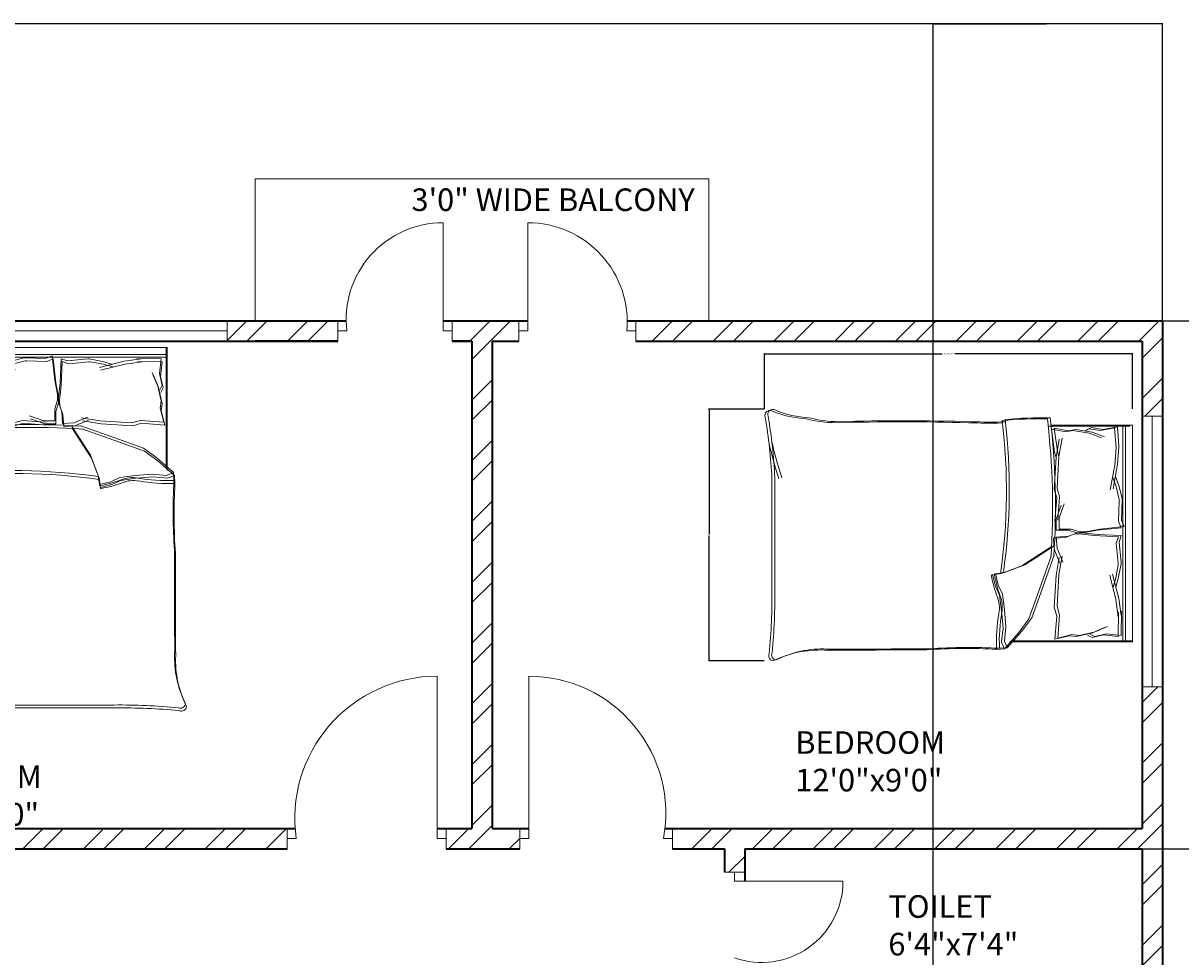
# Model space of a CAD drawing. Units: inches. Extents: x 2165 to 3042, y 1626 to 2968.
# Tile 9 of 11: x 2633 to 2889, y 2191 to 2398. Entities that reach past the tile are written whole.
import ezdxf

# ---------------------------------------------------------------- set-up
doc = ezdxf.new("R2010")
doc.units = ezdxf.units.IN
for name, color, linetype, lineweight in [('A-ANNO-DIMS', 2, 'Continuous', 18), ('A-AREA-IDEN', 7, 'Continuous', 18), ('A-DOOR', 3, 'Continuous', 18), ('A-FLOR-BALC', 7, 'Continuous', 18), ('A-FURN', 8, 'Continuous', 13), ('A-GLAZ', 4, 'Continuous', 18), ('A-WALL', 7, 'Continuous', 35), ('A-WALL-PATT', 252, 'Continuous', 13)]:
    doc.layers.add(name, color=color, linetype=linetype, lineweight=lineweight)
doc.styles.get("Standard").update_dxf_attribs({"font": 'arial.ttf'})
doc.dimstyles.get("Standard").update_dxf_attribs({"dimtxt": 0.18, "dimasz": 0.18, "dimexe": 0.18, "dimexo": 0.0625, "dimgap": 0.09, "dimtad": 0, "dimtih": 1, "dimtoh": 1, "dimdec": 4, "dimzin": 0, "dimdsep": 46, "dimtxsty": 'Standard', "dimcen": 0.09, "dimadec": 0, "dimazin": 0, "dimtfac": 1, "dimtdec": 4, "dimtofl": 0, "dimtmove": 0, "dimatfit": 3, "dimfxl": 1, "dimtolj": 1, "dimtzin": 0, "dimarcsym": 0})

# ---------------------------------------------------------------- blocks, each defined once
blk = doc.blocks.new('BED-DOUBLE')
for p, q in [((0, 51.27), (0, 51.49)), ((0, 51.49), (0.64, 51.49)), ((0.64, 51.49), (27.25, 51.49)), ((0.64, 51.49), (27.25, 51.49)), ((2.17, 3.7), (2.17, 51.49)), ((2.17, 3.7), (2.17, 51.49)), ((27.75, 52.87), (24.5, 49.16)), ((27.75, 52.87), (24.5, 49.16)), ((28.39, 53.1), (25.14, 49.39)), ((28.39, 53.1), (25.14, 49.39)), ((29.49, 52.95), (27.75, 52.87, 3.87)), ((29.49, 52.95), (27.75, 52.87, 3.87)), ((28.37, 51.33), (27.75, 52.87)), ((28.37, 51.33), (27.75, 52.87)), ((28.06, 48.23), (28.37, 51.33)), ((28.06, 48.23), (28.37, 51.33)), ((30.13, 53.18), (28.39, 53.1, 3.87)), ((30.13, 53.18), (28.39, 53.1, 3.87)), ((29, 51.56), (28.39, 53.1)), ((29, 51.56), (28.39, 53.1)), ((28.7, 48.46), (29, 51.56)), ((28.7, 48.46), (29, 51.56)), ((0, 51.27), (26.61, 51.27)), ((0, 51.27), (26.61, 51.27)), ((0, 51.27), (0, 3.48)), ((1.53, 3.48), (1.53, 51.27)), ((1.53, 3.47), (1.53, 51.27)), ((2.56, 50.11), (2.46, 44.71)), ((2.56, 50.11), (2.46, 44.71)), ((2.56, 50.11), (5.77, 49.73)), ((2.56, 50.11), (5.77, 49.73)), ((3.2, 50.34), (3.1, 44.94)), ((3.2, 50.34), (3.1, 44.94)), ((3.2, 50.34), (6.41, 49.96)), ((3.2, 50.34), (6.41, 49.96)), ((8.26, 49.31), (5.58, 48.13)), ((8.26, 49.31), (5.58, 48.13)), ((5.77, 49.73), (8.34, 50.33)), ((5.77, 49.73), (8.34, 50.33)), ((8.9, 49.54), (6.22, 48.36)), ((8.9, 49.54), (6.22, 48.36)), ((6.41, 49.96), (8.98, 50.56)), ((6.41, 49.96), (8.98, 50.56)), ((11.83, 50.11), (8.26, 49.31)), ((11.83, 50.11), (8.26, 49.31)), ((8.34, 50.33), (9.38, 49.81)), ((8.34, 50.33), (9.38, 49.81)), ((12.47, 50.34), (8.9, 49.54)), ((12.47, 50.34), (8.9, 49.54)), ((8.98, 50.56), (10.02, 50.04)), ((8.98, 50.56), (10.02, 50.04)), ((13.43, 49.92), (11.83, 50.11)), ((13.43, 49.92), (11.83, 50.11)), ((14.07, 50.15), (12.47, 50.34)), ((14.07, 50.15), (12.47, 50.34)), ((16.57, 50.7), (13.43, 49.92)), ((16.57, 50.7), (13.43, 49.92)), ((17.21, 50.93), (14.07, 50.15)), ((17.21, 50.93), (14.07, 50.15)), ((16.17, 45.57), (16.57, 50.7)), ((16.17, 45.57), (16.57, 50.7)), ((16.81, 45.79), (17.21, 50.93)), ((16.81, 45.79), (17.21, 50.93)), ((24.5, 49.16), (22.33, 46.22)), ((24.5, 49.16), (22.33, 46.22)), ((25.14, 49.39), (22.97, 46.45)), ((25.14, 49.39), (22.97, 46.45)), ((22.33, 46.22), (20.32, 40.64)), ((22.33, 46.22), (20.32, 40.64)), ((22.97, 46.45), (20.96, 40.87)), ((22.97, 46.45), (20.96, 40.87)), ((28.37, 44.36), (28.06, 48.23)), ((28.37, 44.36), (28.06, 48.23)), ((29, 44.59), (28.7, 48.46)), ((29, 44.59), (28.7, 48.46)), ((2.46, 44.71), (2.54, 45.71)), ((2.46, 44.71), (2.54, 45.71)), ((2.54, 45.71), (3.07, 41.91)), ((2.54, 45.71), (3.07, 41.91)), ((3.1, 44.94), (3.18, 45.94)), ((3.1, 44.94), (3.18, 45.94)), ((3.18, 45.94), (3.71, 42.14)), ((3.18, 45.94), (3.71, 42.14)), ((16.73, 43.61), (16.17, 45.57)), ((16.73, 43.61), (16.17, 45.57)), ((16.3, 36.6), (16.73, 43.61)), ((16.3, 36.6), (16.73, 43.61)), ((17.37, 43.83), (16.81, 45.79)), ((17.37, 43.83), (16.81, 45.79)), ((16.93, 36.82), (17.37, 43.83)), ((16.93, 36.82), (17.37, 43.83)), ((28.83, 40.95), (28.37, 44.36)), ((28.83, 40.95), (28.37, 44.36)), ((29.47, 41.18), (29, 44.59)), ((29.47, 41.18), (29, 44.59)), ((3.07, 41.91), (4.42, 36.5)), ((3.07, 41.91), (4.42, 36.49)), ((3.71, 42.14), (5.06, 36.72)), ((3.71, 42.14), (5.06, 36.72)), ((30.4, 39.17), (29.47, 41.18)), ((30.4, 39.17), (29.47, 41.18)), ((3.67, 39.2), (3.08, 37.14)), ((3.67, 39.2), (3.08, 37.13)), ((4.31, 39.43), (3.72, 37.36)), ((4.31, 39.43), (3.72, 37.36)), ((20.32, 40.64), (17.38, 32.31)), ((20.32, 40.64), (17.38, 32.31)), ((20.96, 40.87), (18.02, 32.53)), ((20.96, 40.87), (18.02, 32.53)), ((29.76, 38.94), (28.83, 40.95)), ((29.76, 38.94), (28.83, 40.95)), ((30.38, 36.46), (29.76, 38.94)), ((30.38, 36.46), (29.76, 38.94)), ((31.02, 36.69), (30.4, 39.17)), ((31.02, 36.69), (30.4, 39.17)), ((79.25, 15.06), (79.25, 39.68)), ((79.25, 15.06), (79.25, 39.68)), ((79.88, 15.29), (79.88, 39.91)), ((79.88, 15.29), (79.88, 39.91)), ((3.08, 37.14), (2.54, 34.2)), ((3.08, 37.13), (2.54, 34.2)), ((3.72, 37.36), (3.18, 34.43)), ((3.72, 37.36), (3.18, 34.43)), ((15.63, 32.56), (16.3, 36.6)), ((15.63, 32.56), (16.3, 36.6)), ((16.27, 32.79), (16.93, 36.82)), ((16.27, 32.79), (16.93, 36.82)), ((23.88, 34.45), (28.37, 36.15)), ((23.88, 34.45), (28.37, 36.15)), ((24.52, 34.68), (29, 36.38)), ((24.52, 34.68), (29, 36.38)), ((28.37, 36.15), (30.38, 36.46)), ((28.37, 36.15), (30.38, 36.46)), ((29, 36.38), (31.02, 36.69)), ((29, 36.38), (31.02, 36.69)), ((2.54, 34.2), (2.56, 33.88)), ((2.54, 34.2), (2.56, 33.88)), ((2.56, 33.88), (2.98, 29.46)), ((2.56, 33.88), (2.98, 29.46)), ((3.18, 34.43), (3.2, 34.11)), ((3.18, 34.43), (3.2, 34.11)), ((3.2, 34.11), (3.62, 29.68)), ((3.2, 34.11), (3.62, 29.68)), ((16.74, 30.75), (15.46, 33.82)), ((16.74, 30.75), (15.46, 33.82)), ((17.38, 30.98), (16.09, 34.05)), ((17.38, 30.98), (16.09, 34.05)), ((17.38, 30.26), (23.88, 34.45)), ((17.38, 30.26), (23.88, 34.45)), ((18.02, 30.49), (24.52, 34.68)), ((18.02, 30.49), (24.52, 34.68)), ((17.53, 28.53), (17.38, 30.98)), ((17.53, 28.53), (17.38, 30.98)), ((2.98, 29.46), (2.49, 27.98)), ((2.98, 29.46), (2.49, 27.98)), ((3.62, 29.68), (3.13, 28.21)), ((3.62, 29.68), (3.13, 28.21)), ((13.02, 27.66), (14.86, 28.36)), ((13.02, 27.66), (14.86, 28.36)), ((14.22, 28.13), (16.89, 28.3)), ((14.22, 28.13), (16.89, 28.3)), ((14.86, 28.36), (17.53, 28.53)), ((14.86, 28.36), (17.53, 28.53)), ((16.89, 28.3), (16.74, 30.75)), ((16.89, 28.3), (16.74, 30.75)), ((1.87, 25.98), (7.22, 26.56)), ((1.87, 25.98), (7.22, 26.56)), ((2.45, 24.54), (1.87, 25.98)), ((2.45, 24.54), (1.87, 25.98)), ((2.49, 27.98), (7.87, 27.73)), ((2.49, 27.98), (7.87, 27.73)), ((2.51, 26.21), (7.86, 26.79)), ((2.51, 26.21), (7.86, 26.79)), ((3.09, 24.77), (2.51, 26.21)), ((3.09, 24.77), (2.51, 26.21)), ((3.13, 28.21), (8.51, 27.96)), ((3.13, 28.21), (8.51, 27.96)), ((7.22, 26.56), (10.4, 27.14)), ((7.22, 26.56), (10.4, 27.14)), ((7.86, 26.79), (11.04, 27.37)), ((7.86, 26.79), (11.04, 27.37)), ((7.87, 27.73), (11.08, 27.35)), ((7.87, 27.73), (11.08, 27.35)), ((8.51, 27.96), (11.72, 27.58)), ((8.51, 27.96), (11.72, 27.58)), ((10.4, 27.14), (11.7, 27.14)), ((10.4, 27.14), (11.7, 27.14)), ((11.04, 27.37), (12.34, 27.37)), ((11.04, 27.37), (12.34, 27.37)), ((11.08, 27.35), (12.38, 27.44)), ((11.08, 27.35), (12.38, 27.44)), ((11.7, 27.14), (13.58, 26.56)), ((11.7, 27.14), (13.58, 26.56)), ((11.72, 27.58), (13.02, 27.66)), ((11.72, 27.58), (13.02, 27.66)), ((12.34, 27.37), (14.22, 26.79)), ((12.34, 27.37), (14.22, 26.79)), ((12.38, 27.44), (14.22, 28.13)), ((12.38, 27.44), (14.22, 28.13)), ((13.58, 26.56), (16.26, 26.56)), ((13.58, 26.56), (16.26, 26.56)), ((14.22, 26.79), (16.9, 26.79)), ((14.22, 26.79), (16.9, 26.79)), ((16.26, 26.56), (16.26, 24.1)), ((16.26, 26.56), (16.26, 24.1)), ((16.9, 26.79), (16.9, 24.33)), ((16.9, 26.79), (16.9, 24.33)), ((2.3, 20.09), (2.45, 24.54)), ((2.3, 20.09), (2.45, 24.54)), ((2.94, 20.32), (3.09, 24.77)), ((2.94, 20.32), (3.09, 24.77)), ((16.26, 24.1), (15.17, 20.96)), ((16.26, 24.1), (15.17, 20.96)), ((16.9, 24.33), (15.81, 21.19)), ((16.9, 24.33), (15.81, 21.19)), ((16.17, 19.38), (16.57, 24.52)), ((16.17, 19.38), (16.57, 24.52)), ((16.81, 19.61), (17.21, 24.74)), ((16.81, 19.61), (17.21, 24.74)), ((2.3, 19.77), (2.3, 20.09)), ((2.3, 19.77), (2.3, 20.09)), ((3.03, 16.88), (2.3, 19.77)), ((3.03, 16.88), (2.3, 19.77)), ((2.94, 20), (2.94, 20.32)), ((2.94, 20), (2.94, 20.32)), ((3.67, 17.11), (2.94, 20)), ((3.67, 17.11), (2.94, 20)), ((16.73, 17.42), (16.17, 19.38)), ((16.73, 17.42), (16.17, 19.38)), ((17.37, 17.65), (16.81, 19.61)), ((17.37, 17.65), (16.81, 19.61)), ((3.75, 14.85), (3.03, 16.88)), ((3.75, 14.85), (3.03, 16.88)), ((3.32, 12.11), (4.33, 17.6)), ((3.32, 12.11), (4.33, 17.6)), ((4.39, 15.08), (3.67, 17.11)), ((4.39, 15.08), (3.67, 17.11)), ((3.96, 12.34), (4.97, 17.83)), ((3.96, 12.34), (4.97, 17.83)), ((16.3, 10.41), (16.73, 17.42)), ((16.3, 10.41), (16.73, 17.42)), ((16.93, 10.64), (17.37, 17.65)), ((16.93, 10.64), (17.37, 17.65)), ((3.03, 8.28), (3.32, 12.11)), ((3.03, 8.28), (3.32, 12.11)), ((3.67, 8.51), (3.96, 12.34)), ((3.67, 8.51), (3.96, 12.34)), ((15.63, 6.38), (16.3, 10.41)), ((15.63, 6.38), (16.3, 10.41)), ((16.27, 6.61), (16.93, 10.64)), ((16.27, 6.61), (16.93, 10.64)), ((16.3, 10.41), (16.62, 9.28)), ((16.3, 10.41), (16.62, 9.28)), ((16.93, 10.64), (17.26, 9.51)), ((16.93, 10.64), (17.26, 9.51)), ((3.01, 8.18), (3.03, 8.28)), ((3.01, 8.18), (3.03, 8.28)), ((3.34, 3.9), (3.01, 8.18)), ((3.34, 3.9), (3.01, 8.18)), ((3.65, 8.41), (3.67, 8.51)), ((3.65, 8.41), (3.67, 8.51)), ((3.98, 4.13), (3.65, 8.41)), ((3.98, 4.13), (3.65, 8.41)), ((16.62, 9.28), (17.34, 4.18)), ((16.62, 9.28), (17.34, 4.18)), ((17.26, 9.51), (17.98, 4.41)), ((17.26, 9.51), (17.98, 4.41)), ((8.96, 5.05), (6.21, 6.06)), ((8.96, 5.05), (6.21, 6.06)), ((9.59, 5.28), (6.85, 6.29)), ((9.59, 5.28), (6.85, 6.29)), ((13.21, 4.7), (9.59, 5.28)), ((13.21, 4.7), (9.59, 5.28)), ((18.11, 3.48), (0, 3.48)), ((18.11, 3.47), (0, 3.47)), ((18.75, 3.7), (0.64, 3.7)), ((18.75, 3.7), (0.64, 3.7)), ((3.32, 3.89), (6.5, 4.47)), ((3.32, 3.89), (6.5, 4.47)), ((3.96, 4.12), (7.14, 4.7)), ((3.96, 4.12), (7.14, 4.7)), ((6.5, 4.47), (9.1, 4.04)), ((6.5, 4.47), (9.1, 4.04)), ((7.14, 4.7), (9.74, 4.27)), ((7.14, 4.7), (9.74, 4.27)), ((12.57, 4.47), (8.96, 5.05)), ((12.57, 4.47), (8.96, 5.05)), ((9.1, 4.04), (10.11, 4.62)), ((9.1, 4.04), (10.11, 4.62)), ((9.74, 4.27), (10.75, 4.85)), ((9.74, 4.27), (10.75, 4.85)), ((14.16, 4.76), (12.57, 4.47)), ((14.16, 4.76), (12.57, 4.47)), ((14.8, 4.99), (13.21, 4.7)), ((14.8, 4.99), (13.21, 4.7)), ((17.34, 4.18), (14.16, 4.76)), ((17.34, 4.18), (14.16, 4.76)), ((17.98, 4.41), (14.8, 4.99)), ((17.98, 4.41), (14.8, 4.99))]:
    blk.add_line(p, q)
for centre, radius, start, end in [((68.67, 76.16), 23.07, 267.4714, 296.4681), ((68.67, 76.16), 23.07, 267.4714, 296.4681), ((69.31, 76.39), 23.07, 267.4714, 296.4681), ((69.31, 76.39), 23.07, 267.4714, 296.4681), ((78.87, 54.41), 1.1, 332.6588, 86.02), ((78.87, 54.41), 1.1, 332.6588, 86.02), ((212.28, 41.15), 133.04, 174.4998, 180.6351), ((212.28, 41.15), 133.04, 174.4998, 180.6351), ((79.51, 54.64), 1.1, 332.6588, 86.02), ((79.51, 54.64), 1.1, 332.6588, 86.02), ((212.92, 41.38), 133.04, 174.4998, 180.6351), ((212.92, 41.38), 133.04, 174.4998, 180.6351), ((-6.66, 51.33), 36.18, 349.8763, 2.5657), ((-6.66, 51.33), 36.18, 349.8763, 2.5657), ((36.32, 182.27), 129.5, 266.9791, 273.8365), ((36.32, 182.27), 129.5, 266.9791, 273.8365), ((-6.02, 51.56), 36.18, 349.8763, 2.5657), ((-6.02, 51.56), 36.18, 349.8763, 2.5657), ((36.95, 182.49), 129.5, 266.9791, 273.8365), ((36.95, 182.49), 129.5, 266.9791, 273.8365), ((67.82, -4508.74), 4561.86, 90.00217, 90.28689), ((67.82, -4508.74), 4561.86, 90.00217, 90.28689), ((68.46, -4508.52), 4561.86, 90.00217, 90.28689), ((68.46, -4508.52), 4561.86, 90.00217, 90.28689), ((35.07, 43.74), 6.22, 168.6608, 203.7384), ((35.07, 43.74), 6.22, 168.6608, 203.7384), ((35.71, 43.97), 6.22, 168.6608, 203.7384), ((35.71, 43.97), 6.22, 168.6608, 203.7384), ((1.48, 31.15), 29.65, 10.6617, 19.8806), ((1.48, 31.15), 29.65, 10.6617, 19.8806), ((2.12, 31.38), 29.65, 10.6617, 19.8806), ((2.12, 31.38), 29.65, 10.6617, 19.8806), ((156.32, 17.76), 129.02, 171.7845, 186.9006), ((156.32, 17.76), 129.02, 171.7845, 186.9006), ((156.96, 17.98), 129.02, 171.7845, 186.9006), ((156.96, 17.98), 129.02, 171.7845, 186.9006), ((30.44, 36.64), 0.185, 250.2464, 1.1377), ((30.44, 36.64), 0.185, 250.2464, 1.1377), ((31.08, 36.86), 0.185, 250.2464, 1.1377), ((31.08, 36.86), 0.185, 250.2464, 1.1377), ((182.05, 21.36), 164.97, 176.0865, 186.7821), ((182.05, 21.36), 164.97, 176.0865, 186.7821), ((182.69, 21.59), 164.97, 176.0865, 186.7821), ((182.69, 21.59), 164.97, 176.0865, 186.7821), ((-23.71, -17.22), 106.46, 13.3832, 17.7053), ((-23.71, -17.22), 106.46, 13.3832, 17.7053), ((-23.07, -16.99), 106.46, 13.3832, 17.7053), ((-23.07, -16.99), 106.46, 13.3832, 17.7053), ((200.84, 21.43), 121.76, 182.9958, 189.4091), ((200.84, 21.43), 121.76, 182.9958, 189.4091), ((201.48, 21.66), 121.76, 182.9958, 189.4091), ((201.48, 21.65), 121.76, 182.9958, 189.4091), ((31.17, -167.31), 170.11, 88.4762, 91.0082), ((31.17, -167.31), 170.11, 88.4762, 91.0082), ((31.81, -167.08), 170.11, 88.4762, 91.0082), ((31.81, -167.08), 170.11, 88.4762, 91.0082), ((50.61, 484.82), 482.31, 268.2277, 271.7185), ((50.61, 484.82), 482.31, 268.2277, 271.7185), ((51.25, 485.05), 482.31, 268.2277, 271.7185), ((51.25, 485.05), 482.31, 268.2277, 271.7185), ((64.52, -26.9), 29.63, 76.0648, 88.9113), ((64.52, -26.9), 29.63, 76.0648, 88.9113), ((65.15, -26.67), 29.63, 76.0648, 88.9113), ((65.15, -26.67), 29.63, 76.0648, 88.9113), ((20.1, 85.16), 83.31, 268.7218, 275.604), ((20.1, 85.16), 83.31, 268.7218, 275.604), ((20.74, 85.39), 83.31, 268.7218, 275.604), ((20.74, 85.39), 83.31, 268.7218, 275.604), ((70.28, -21.66), 23.56, 67.9751, 86.652), ((70.28, -21.66), 23.56, 67.9751, 86.652), ((70.92, -21.43), 23.56, 67.9751, 86.652), ((70.92, -21.43), 23.56, 67.9751, 86.652), ((79.72, 1.09), 1.09, 236.1736, 23.4781), ((79.72, 1.09), 1.09, 236.1736, 23.4781), ((80.36, 1.32), 1.09, 236.1736, 23.4781), ((80.36, 1.32), 1.09, 236.1736, 23.4781)]:
    blk.add_arc(centre, radius, start, end)
blk = doc.blocks.new('BALCONY-RAIL-PLAN')
for p, q in [((0, 31.5), (0, 0)), ((100.5, 31.5), (100.5, 0)), ((100.5, 0), (0, 0))]:
    blk.add_line(p, q)
blk = doc.blocks.new('WIN-60-A')
for p, q in [((4.5, 60), (0, 60)), ((0, 60), (2.25, 60)), ((2.25, 60), (2.25, 0)), ((2.25, 0), (0, 0)), ((0, 0), (4.5, 0))]:
    blk.add_line(p, q)
blk = doc.blocks.new('WIN-60-B')
for p, q in [((0, 4.5), (0, 0)), ((60, 2.25), (60, 4.5)), ((60, 4.5), (60, 0)), ((0, 0), (0, 2.25)), ((0, 2.25), (60, 2.25))]:
    blk.add_line(p, q)
blk = doc.blocks.new('*D18')
at = {"layer": 'A-ANNO-DIMS', "color": 0, "lineweight": -2, "transparency": 16777216}
for p, q in [((2796.96, 2312.6), (2796.96, 2324.95)), ((2797.14, 2324.77), (2836.36, 2324.77)), ((2878.32, 2324.77), (2839.1, 2324.77)), ((2878.5, 2312.6), (2878.5, 2324.95))]:
    blk.add_line(p, q, dxfattribs=at)
at = {"layer": 'A-ANNO-DIMS', "color": 0, "transparency": 16777216}
for points in [[(2797.14, 2324.8), (2797.14, 2324.74), (2796.96, 2324.77)], [(2878.32, 2324.8), (2878.32, 2324.74), (2878.5, 2324.77)]]:
    blk.add_solid(points, dxfattribs=at)
at = {"layer": 'Defpoints', "color": 0, "transparency": 16777216}
for p in [(2796.96, 2324.77), (2796.96, 2312.54), (2878.5, 2312.54)]:
    blk.add_point(p, dxfattribs=at)
at = {"layer": 'A-ANNO-DIMS', "color": 0, "transparency": 16777216, "insert": (2837.73, 2324.77), "char_height": 0.18, "attachment_point": 5}
blk.add_mtext('\\A1;DOUBLE BED 82 TYP.', dxfattribs=at)
blk = doc.blocks.new('*D19')
at = {"layer": 'A-ANNO-DIMS', "color": 0, "lineweight": -2, "transparency": 16777216}
for p, q in [((2796.89, 2312.54), (2784.54, 2312.54)), ((2784.72, 2312.36), (2784.72, 2284.81)), ((2784.72, 2256.89), (2784.72, 2284.44)), ((2796.89, 2256.71), (2784.54, 2256.71))]:
    blk.add_line(p, q, dxfattribs=at)
at = {"layer": 'A-ANNO-DIMS', "color": 0, "transparency": 16777216}
for points in [[(2784.69, 2312.36), (2784.75, 2312.36), (2784.72, 2312.54)], [(2784.69, 2256.89), (2784.75, 2256.89), (2784.72, 2256.71)]]:
    blk.add_solid(points, dxfattribs=at)
at = {"layer": 'Defpoints', "color": 0, "transparency": 16777216}
for p in [(2796.96, 2312.54), (2784.72, 2256.71), (2796.96, 2256.71)]:
    blk.add_point(p, dxfattribs=at)
at = {"layer": 'A-ANNO-DIMS', "color": 0, "transparency": 16777216, "insert": (2784.72, 2284.62), "char_height": 0.18, "attachment_point": 5}
blk.add_mtext('\\A1;56 TYP.', dxfattribs=at)
blk = doc.blocks.new('*D50')
at = {"layer": 'A-ANNO-DIMS', "color": 0, "lineweight": -2, "transparency": 16777216}
for p, q in [((2286.6, 2332.14), (2286.6, 2398.06)), ((2885.1, 2332.14), (2885.1, 2398.06)), ((2286.78, 2397.88), (2585.46, 2397.88)), ((2884.92, 2397.88), (2586.25, 2397.88))]:
    blk.add_line(p, q, dxfattribs=at)
at = {"layer": 'A-ANNO-DIMS', "color": 0, "transparency": 16777216}
for points in [[(2286.78, 2397.91), (2286.78, 2397.85), (2286.6, 2397.88)], [(2884.92, 2397.91), (2884.92, 2397.85), (2885.1, 2397.88)]]:
    blk.add_solid(points, dxfattribs=at)
at = {"layer": 'Defpoints', "color": 0, "transparency": 16777216}
for p in [(2885.1, 2397.88), (2286.6, 2332.08), (2885.1, 2332.08)]:
    blk.add_point(p, dxfattribs=at)
at = {"layer": 'A-ANNO-DIMS', "color": 0, "transparency": 16777216, "insert": (2585.85, 2397.88), "char_height": 0.18, "attachment_point": 5}
blk.add_mtext('\\A1;598.5', dxfattribs=at)
blk = doc.blocks.new('*D61')
at = {"layer": 'A-ANNO-DIMS', "color": 0, "lineweight": -2, "transparency": 16777216}
for p, q in [((2880.67, 2215.08), (2919.58, 2215.08)), ((2919.4, 2214.9), (2919.4, 2175.01)), ((2919.4, 2134.76), (2919.4, 2174.65)), ((2885.17, 2134.58), (2919.58, 2134.58))]:
    blk.add_line(p, q, dxfattribs=at)
at = {"layer": 'A-ANNO-DIMS', "color": 0, "transparency": 16777216}
for points in [[(2919.37, 2214.9), (2919.43, 2214.9), (2919.4, 2215.08)], [(2919.37, 2134.76), (2919.43, 2134.76), (2919.4, 2134.58)]]:
    blk.add_solid(points, dxfattribs=at)
at = {"layer": 'Defpoints', "color": 0, "transparency": 16777216}
for p in [(2880.6, 2215.08), (2919.4, 2215.08), (2885.1, 2134.58)]:
    blk.add_point(p, dxfattribs=at)
at = {"layer": 'A-ANNO-DIMS', "color": 0, "transparency": 16777216, "insert": (2919.4, 2174.83), "char_height": 0.18, "attachment_point": 5}
blk.add_mtext('\\A1;80.5', dxfattribs=at)
blk = doc.blocks.new('*D62')
at = {"layer": 'A-ANNO-DIMS', "color": 0, "lineweight": -2, "transparency": 16777216}
for p, q in [((2885.17, 2332.08), (2919.58, 2332.08)), ((2919.4, 2331.9), (2919.4, 2273.76)), ((2919.4, 2215.26), (2919.4, 2273.4)), ((2880.67, 2215.08), (2919.58, 2215.08))]:
    blk.add_line(p, q, dxfattribs=at)
at = {"layer": 'A-ANNO-DIMS', "color": 0, "transparency": 16777216}
for points in [[(2919.37, 2331.9), (2919.43, 2331.9), (2919.4, 2332.08)], [(2919.37, 2215.26), (2919.43, 2215.26), (2919.4, 2215.08)]]:
    blk.add_solid(points, dxfattribs=at)
at = {"layer": 'Defpoints', "color": 0, "transparency": 16777216}
for p in [(2885.1, 2332.08), (2919.4, 2332.08), (2880.6, 2215.08)]:
    blk.add_point(p, dxfattribs=at)
at = {"layer": 'A-ANNO-DIMS', "color": 0, "transparency": 16777216, "insert": (2919.4, 2273.58), "char_height": 0.18, "attachment_point": 5}
blk.add_mtext('\\A1;117', dxfattribs=at)
blk = doc.blocks.new('*D63')
at = {"layer": 'A-ANNO-DIMS', "color": 0, "lineweight": -2, "transparency": 16777216}
for p, q in [((2834.35, 2075.64), (2834.35, 2398.06)), ((2885.1, 2075.64), (2885.1, 2398.06)), ((2834.53, 2397.88), (2859.34, 2397.88)), ((2884.92, 2397.88), (2860.12, 2397.88))]:
    blk.add_line(p, q, dxfattribs=at)
at = {"layer": 'A-ANNO-DIMS', "color": 0, "transparency": 16777216}
for points in [[(2834.53, 2397.91), (2834.53, 2397.85), (2834.35, 2397.88)], [(2884.92, 2397.91), (2884.92, 2397.85), (2885.1, 2397.88)]]:
    blk.add_solid(points, dxfattribs=at)
at = {"layer": 'Defpoints', "color": 0, "transparency": 16777216}
for p in [(2885.1, 2397.88), (2834.35, 2075.58), (2885.1, 2075.58)]:
    blk.add_point(p, dxfattribs=at)
at = {"layer": 'A-ANNO-DIMS', "color": 0, "transparency": 16777216, "insert": (2859.73, 2397.88), "char_height": 0.18, "attachment_point": 5}
blk.add_mtext('\\A1;50.75', dxfattribs=at)

msp = doc.modelspace()

# ---------------------------------------------------------------- hatches: boundary and pattern name
at = {"layer": 'A-WALL-PATT'}
h = msp.add_hatch(dxfattribs=at)
h.set_pattern_fill('ANSI32', color=256)
h.paths.add_polyline_path([(2406.4931, 2332.0783), (2286.6045, 2332.0783), (2286.6045, 2310.967), (2288.8545, 2310.967), (2291.1045, 2310.967), (2291.1045, 2327.5783), (2406.4931, 2327.5783), (2406.4931, 2329.8283)])
h.paths.add_polyline_path([(2439.6045, 2327.5783), (2444.9584, 2327.5783), (2444.9584, 2332.0783), (2430.2901, 2332.0783), (2430.2901, 2329.8283), (2430.2901, 2327.5783), (2435.1045, 2327.5783), (2435.1045, 2219.5783), (2431.0902, 2219.5783), (2431.0902, 2215.0783), (2435.1045, 2215.0783), (2444.1108, 2215.0783), (2444.1108, 2217.3283), (2444.1108, 2219.5783), (2439.6045, 2219.5783)])
h.paths.add_polyline_path([(2497.5418, 2329.8283), (2497.5418, 2332.0783), (2470.1978, 2332.0783), (2470.1978, 2327.5783), (2497.5418, 2327.5783)])
h.paths.add_polyline_path([(2617.9543, 2332.0783), (2557.5418, 2332.0783), (2557.5418, 2327.5783), (2583.6045, 2327.5783), (2583.6045, 2219.5783), (2474.0523, 2219.5783), (2474.0523, 2215.0783), (2583.6045, 2215.0783), (2583.6045, 2107.0783), (2579.3609, 2107.0783), (2579.3609, 2102.5783), (2588.1045, 2102.5783), (2593.5283, 2102.5783), (2593.5283, 2104.8283), (2593.5283, 2107.0783), (2588.1045, 2107.0783), (2588.1045, 2215.0783), (2691.2325, 2215.0783), (2691.2325, 2217.3283), (2691.2325, 2219.5783), (2588.1045, 2219.5783), (2588.1045, 2327.5783), (2617.9543, 2327.5783)])
h.paths.add_polyline_path([(2702.4444, 2329.8283), (2702.4444, 2332.0783), (2677.9543, 2332.0783), (2677.9543, 2327.5783), (2702.4444, 2327.5783)])
h.paths.add_polyline_path([(2736.6045, 2327.5783), (2742.5161, 2327.5783), (2742.5161, 2329.8283), (2742.5161, 2332.0783), (2727.7639, 2332.0783), (2727.7639, 2329.8283), (2727.7639, 2327.5783), (2732.1045, 2327.5783), (2732.1045, 2219.5783), (2726.4404, 2219.5783), (2726.4404, 2215.0783), (2732.1045, 2215.0783), (2742.7291, 2215.0783), (2742.7291, 2217.3283), (2742.7291, 2219.5783), (2736.6045, 2219.5783)])
h.paths.add_polyline_path([(2885.1045, 2332.0783), (2768.4887, 2332.0783), (2768.4887, 2327.5783), (2784.6045, 2327.5783), (2880.6045, 2327.5783), (2880.6045, 2310.967), (2885.1045, 2310.967)])
h.paths.add_polyline_path([(2885.1045, 2250.967), (2880.6045, 2250.967), (2880.6045, 2219.5783), (2776.5755, 2219.5783), (2776.5755, 2215.0783), (2788.1045, 2215.0783), (2788.1045, 2209.8634), (2790.3545, 2209.8634), (2792.6045, 2209.8634), (2792.6045, 2215.0783), (2880.6045, 2215.0783), (2880.6045, 2139.0783), (2871.2037, 2139.0783), (2871.2037, 2134.5783), (2885.1045, 2134.5783)])
h.paths.add_polyline_path([(2545.013, 2107.0783), (2474.0523, 2107.0783), (2291.1045, 2107.0783), (2291.1045, 2102.5783), (2535.6045, 2102.5783), (2535.6045, 2096.8046), (2537.8545, 2096.8046), (2540.1045, 2096.8046), (2540.1045, 2102.5783), (2545.013, 2102.5783), (2545.013, 2104.8283)])
h.paths.add_polyline_path([(2397.7297, 2217.3283), (2397.7297, 2219.5783), (2291.1045, 2219.5783), (2291.1045, 2250.967), (2286.6045, 2250.967), (2286.6045, 2206.1346), (2288.8545, 2206.1346), (2291.1045, 2206.1346), (2291.1045, 2215.0783), (2367.1045, 2215.0783), (2367.1045, 2212.2868), (2371.6045, 2212.2868), (2371.6045, 2215.0783), (2397.7297, 2215.0783)])
h.paths.add_polyline_path([(2291.1045, 1978.5783), (2367.1045, 1978.5783), (2371.6045, 1978.5783), (2373.2641, 1978.5783), (2374.4883, 1978.5783), (2374.4883, 1980.8283), (2374.4883, 1983.0783), (2371.6045, 1983.0783), (2371.6045, 1986.964), (2369.9051, 1986.964), (2369.3545, 1986.964), (2367.1045, 1986.964), (2367.1045, 1983.0783), (2291.1045, 1983.0783), (2291.1045, 2001.1808), (2286.6045, 2001.1808), (2286.6045, 1947.0203), (2288.8545, 1947.0203), (2291.1045, 1947.0203)])
h.paths.add_polyline_path([(2291.1045, 1887.0203), (2286.6045, 1887.0203), (2286.6045, 1842.0783), (2381.2561, 1842.0783), (2381.2561, 1844.3283), (2381.2561, 1846.5783), (2363.1045, 1846.5783), (2291.1045, 1846.5783)])
h.paths.add_polyline_path([(2415.6045, 1978.5783), (2421.1681, 1978.5783), (2421.1681, 1983.0783), (2415.6045, 1983.0783), (2406.5227, 1983.0783), (2406.5227, 1980.8283), (2406.5227, 1978.5783), (2411.1045, 1978.5783), (2411.1045, 1846.5783), (2406.7549, 1846.5783), (2406.7549, 1842.0783), (2419.2885, 1842.0783), (2419.2885, 1844.3283), (2419.2885, 1846.5783), (2415.6045, 1846.5783)])
h.paths.add_polyline_path([(2586.6045, 1982.779), (2586.6045, 1991.5911), (2582.1045, 1991.5911), (2582.1045, 1982.779), (2540.1045, 1982.779), (2540.1045, 2036.779), (2582.1045, 2036.779), (2582.1045, 2027.6051), (2586.6045, 2027.6051), (2586.6045, 2041.279), (2582.1045, 2041.279), (2540.1045, 2041.279), (2540.1045, 2063.9064), (2537.8545, 2063.9064), (2535.6045, 2063.9064), (2535.6045, 1983.0783), (2455.068, 1983.0783), (2455.068, 1978.5783), (2535.6045, 1978.5783), (2535.6045, 1846.5783), (2522.622, 1846.5783), (2522.622, 1842.0783), (2535.6045, 1842.0783), (2535.6045, 1806.0783), (2535.6045, 1801.5783), (2556.726, 1801.5783), (2556.726, 1803.8283), (2556.726, 1806.0783), (2540.1045, 1806.0783), (2540.1045, 1842.0783), (2540.1045, 1846.5783), (2540.1045, 1978.279), (2586.6045, 1978.279)])
h.paths.add_polyline_path([(2636.1045, 1978.5783), (2717.6642, 1978.5783), (2717.6642, 1980.8283), (2717.6642, 1983.0783), (2636.1045, 1983.0783), (2636.1045, 2063.9064), (2633.8545, 2063.9064), (2631.6045, 2063.9064), (2631.6045, 1846.5783), (2631.6045, 1842.0783), (2631.6045, 1806.0783), (2604.726, 1806.0783), (2604.726, 1801.5783), (2636.1045, 1801.5783), (2636.1045, 1842.0783), (2644.3411, 1842.0783), (2644.3411, 1844.3283), (2644.3411, 1846.5783), (2636.1045, 1846.5783)])
h.paths.add_polyline_path([(2760.6045, 1978.5783), (2764.9931, 1978.5783), (2764.9931, 1983.0783), (2750.4727, 1983.0783), (2750.4727, 1980.8283), (2750.4727, 1978.5783), (2756.1045, 1978.5783), (2756.1045, 1846.5783), (2749.4543, 1846.5783), (2749.4543, 1842.0783), (2765.1894, 1842.0783), (2765.1894, 1846.5783), (2760.6045, 1846.5783)])
h.paths.add_polyline_path([(2880.6045, 1983.0783), (2804.6045, 1983.0783), (2804.6045, 1988.3825), (2802.3545, 1988.3825), (2800.1045, 1988.3825), (2800.1045, 1983.0783), (2800.1045, 1978.5783), (2880.6045, 1978.5783)])
h.paths.add_polyline_path([(2885.1045, 2075.5783), (2871.2037, 2075.5783), (2871.2037, 2071.0783), (2880.6045, 2071.0783), (2880.6045, 1948.8144), (2885.1045, 1948.8144)])
h.paths.add_polyline_path([(2885.1045, 1888.8144), (2880.6045, 1888.8144), (2880.6045, 1846.5783), (2792.1167, 1846.5783), (2792.1167, 1842.0783), (2885.1045, 1842.0783)])
h.paths.add_polyline_path([(2724.4848, 1846.5783), (2708.1045, 1846.5783), (2692.3411, 1846.5783), (2692.3411, 1842.0783), (2724.4848, 1842.0783), (2724.4848, 1844.3283)])
h.paths.add_polyline_path([(2474.622, 1844.4672), (2474.622, 1846.5783), (2444.7417, 1846.5783), (2444.7417, 1842.0783), (2474.622, 1842.0783)])

# ---------------------------------------------------------------- linework, layer by layer
at = {"layer": 'A-DOOR'}
for p, q in [((2725.7639, 2329.8283), (2725.7639, 2353.8283)), ((2744.5161, 2329.8283), (2744.5161, 2353.8283)), ((2702.4444, 2332.0783), (2702.4444, 2327.5783)), ((2727.7639, 2327.5783), (2727.7639, 2332.0783)), ((2727.7639, 2332.0783), (2727.7639, 2329.8283)), ((2742.5161, 2332.0783), (2742.5161, 2327.5783)), ((2768.4887, 2332.0783), (2768.4887, 2327.5783)), ((2702.4444, 2327.5783), (2702.4444, 2329.8283)), ((2702.4444, 2329.8283), (2704.4444, 2329.8283)), ((2727.7639, 2329.8283), (2725.7639, 2329.8283)), ((2742.5161, 2327.5783), (2742.5161, 2329.8283)), ((2742.5161, 2329.8283), (2742.5161, 2329.8283)), ((2742.5161, 2329.8283), (2744.5161, 2329.8283)), ((2768.4887, 2329.8283), (2766.4887, 2329.8283)), ((2768.4887, 2327.5783), (2768.4887, 2329.8283)), ((2724.4404, 2217.3283), (2724.4404, 2253.3283)), ((2744.7291, 2217.3283), (2744.7291, 2253.3283)), ((2691.2325, 2219.5783), (2691.2325, 2215.0783)), ((2726.4404, 2219.5783), (2726.4404, 2215.0783)), ((2742.7291, 2219.5783), (2742.7291, 2215.0783)), ((2776.5755, 2219.5783), (2776.5755, 2215.0783)), ((2691.2325, 2215.0783), (2691.2325, 2217.3283)), ((2691.2325, 2217.3283), (2693.2325, 2217.3283)), ((2726.4404, 2217.3283), (2724.4404, 2217.3283)), ((2726.4404, 2215.0783), (2726.4404, 2217.3283)), ((2742.7291, 2215.0783), (2742.7291, 2217.3283)), ((2742.7291, 2217.3283), (2744.7291, 2217.3283)), ((2776.5755, 2217.3283), (2774.5755, 2217.3283)), ((2776.5755, 2215.0783), (2776.5755, 2217.3283)), ((2792.6045, 2209.8634), (2788.1045, 2209.8634)), ((2788.1045, 2209.8634), (2790.3545, 2209.8634)), ((2790.3545, 2209.8634), (2790.3545, 2207.8634)), ((2790.3545, 2207.8634), (2814.3545, 2207.8634))]:
    msp.add_line(p, q, dxfattribs=at)
for centre, radius, start, end in [((2725.7639, 2332.3591), 21.4692, 90, 186.769799), ((2744.5161, 2331.7701), 22.0582, 354.949806, 90), ((2724.4404, 2221.8015), 31.5268, 90, 188.156957), ((2744.7291, 2222.956), 30.3723, 349.322009, 90), ((2796.3519, 2207.8634), 18.0025, 250.540061, 0)]:
    msp.add_arc(centre, radius, start, end, dxfattribs=at)
at = {"layer": 'A-WALL'}
for p, q in [((2468.4837, 2332.0783), (2704.2966, 2332.0783)), ((2468.4837, 2332.0783), (2704.2966, 2332.0783)), ((2725.7639, 2332.0783), (2744.5161, 2332.0783)), ((2725.7639, 2332.0783), (2744.5161, 2332.0783)), ((2766.5722, 2332.0783), (2885.1045, 2332.0783)), ((2766.5722, 2332.0783), (2885.1045, 2332.0783)), ((2885.1045, 2332.0783), (2885.1045, 2134.5783)), ((2588.1045, 2327.5783), (2702.4444, 2327.5783)), ((2702.4444, 2327.5783), (2684.1045, 2327.5783)), ((2732.1045, 2327.5783), (2727.7639, 2327.5783)), ((2727.7639, 2327.5783), (2732.1045, 2327.5783)), ((2732.1045, 2327.5783), (2732.1045, 2219.5783)), ((2736.6045, 2327.5783), (2736.6045, 2219.5783)), ((2736.6045, 2327.5783), (2742.5161, 2327.5783)), ((2736.6045, 2327.5783), (2742.5161, 2327.5783)), ((2768.4887, 2327.5783), (2784.6045, 2327.5783)), ((2768.4887, 2327.5783), (2880.6045, 2327.5783)), ((2880.6045, 2327.5783), (2880.6045, 2219.5783)), ((2588.1045, 2219.5783), (2692.992, 2219.5783)), ((2724.4404, 2219.5783), (2732.1045, 2219.5783)), ((2736.6045, 2219.5783), (2744.7291, 2219.5783)), ((2774.913, 2219.5783), (2880.6045, 2219.5783)), ((2588.1045, 2215.0783), (2691.2325, 2215.0783)), ((2726.4404, 2215.0783), (2732.1045, 2215.0783)), ((2732.1045, 2215.0783), (2742.7291, 2215.0783)), ((2776.5755, 2215.0783), (2788.1045, 2215.0783)), ((2788.1045, 2215.0783), (2788.1045, 2209.8634)), ((2792.6045, 2215.0783), (2792.6045, 2207.8634)), ((2792.6045, 2215.0783), (2880.6045, 2215.0783)), ((2880.6045, 2215.0783), (2880.6045, 2139.0783))]:
    msp.add_line(p, q, dxfattribs=at)

# ---------------------------------------------------------------- block references
at = {"layer": 'A-FLOR-BALC', "rotation": 180}
msp.add_blockref('BALCONY-RAIL-PLAN', (2784.6049, 2363.5786), dxfattribs=at)
at = {"layer": 'A-FURN'}
for p, rotation in [((2613.1768, 2326.1825), 269.9999998332427), ((2878.5051, 2312.4496), 180)]:
    msp.add_blockref('BED-DOUBLE', p, dxfattribs=dict(at, rotation=rotation))
at = {"layer": 'A-GLAZ', "extrusion": (0, 0, -1), "zscale": -1, "rotation": 180}
msp.add_blockref('WIN-60-B', (-2617.9544, 2332.0786), dxfattribs=at)
at = {"layer": 'A-GLAZ', "rotation": 180}
msp.add_blockref('WIN-60-A', (2885.1049, 2310.967), dxfattribs=at)

# ---------------------------------------------------------------- texts
at = {"layer": 'A-AREA-IDEN', "char_height": 5, "attachment_point": 1}
for s, width, insert in [('3\'0" WIDE BALCONY', 69.420923, (2718.7607, 2361.4202)), ('BEDROOM\\P12\'0"x9\'0"', 146.554554, (2803.7832, 2241.1212)), ('BEDROOM\\P12\'0"x9\'0"', 99.842091, (2603.6657, 2233.5451)), ('TOILET\\P6\'4"x7\'4"', 98.170183, (2824.3966, 2204.7714))]:
    msp.add_mtext_dynamic_manual_height_columns(s, width=width, gutter_width=12.5, heights=[0], dxfattribs=dict(at, insert=insert))

# ---------------------------------------------------------------- dimensions: what is measured, and where the dimension line sits
at = {"layer": 'A-ANNO-DIMS'}
for p1, p2, override, picture, middle in [((2286.6045, 2332.0783), (2885.1045, 2332.0783), {"dimdec": 1, "dimlfac": 1, "dimrnd": 0, "dimzin": 0, "dimdsep": 46, "dimlunit": 2}, '*D50', (2585.8545, 2397.8783)), ((2834.3545, 2075.5783), (2885.1045, 2075.5783), {"dimdec": 2, "dimlfac": 1, "dimrnd": 0, "dimzin": 0, "dimdsep": 46, "dimlunit": 2}, '*D63', (2859.7295, 2397.8783))]:
    dim = msp.add_linear_dim(base=(2885.1045, 2397.8783), p1=p1, p2=p2, dimstyle='Standard', override=override, dxfattribs=at)
    dim.commit()
    dim.dimension.update_dxf_attribs({"geometry": picture, "text_midpoint": middle})
for base, p1, p2, override, picture, middle in [((2919.4045, 2332.0783), (2880.6045, 2215.0783), (2885.1045, 2332.0783), {"dimdec": 0, "dimlfac": 1, "dimrnd": 0, "dimzin": 0, "dimdsep": 46, "dimlunit": 2}, '*D62', (2919.4045, 2273.5783)), ((2919.4045, 2215.0783), (2885.1045, 2134.5783), (2880.6045, 2215.0783), {"dimdec": 1, "dimlfac": 1, "dimrnd": 0, "dimzin": 0, "dimdsep": 46, "dimlunit": 2}, '*D61', (2919.4045, 2174.8283))]:
    dim = msp.add_linear_dim(base=base, p1=p1, p2=p2, angle=90, dimstyle='Standard', override=override, dxfattribs=at)
    dim.commit()
    dim.dimension.update_dxf_attribs({"geometry": picture, "text_midpoint": middle})
for base, p1, p2, angle, text, picture, middle in [((2796.956, 2324.7683), (2878.5046, 2312.5361), (2796.956, 2312.5361), 180, 'DOUBLE BED <> TYP.', '*D18', (2837.7303, 2324.7683)), ((2784.7237, 2256.7115), (2796.956, 2312.5361), (2796.956, 2256.7115), 270, '<> TYP.', '*D19', (2784.7237, 2284.6238))]:
    dim = msp.add_linear_dim(base=base, p1=p1, p2=p2, angle=angle, text=text, dimstyle='Standard', override={"dimdec": 0, "dimlfac": 1, "dimrnd": 0, "dimzin": 0, "dimdsep": 46, "dimlunit": 2}, dxfattribs=at)
    dim.commit()
    dim.dimension.update_dxf_attribs({"geometry": picture, "text_midpoint": middle})

doc.saveas('drawing.dxf')
